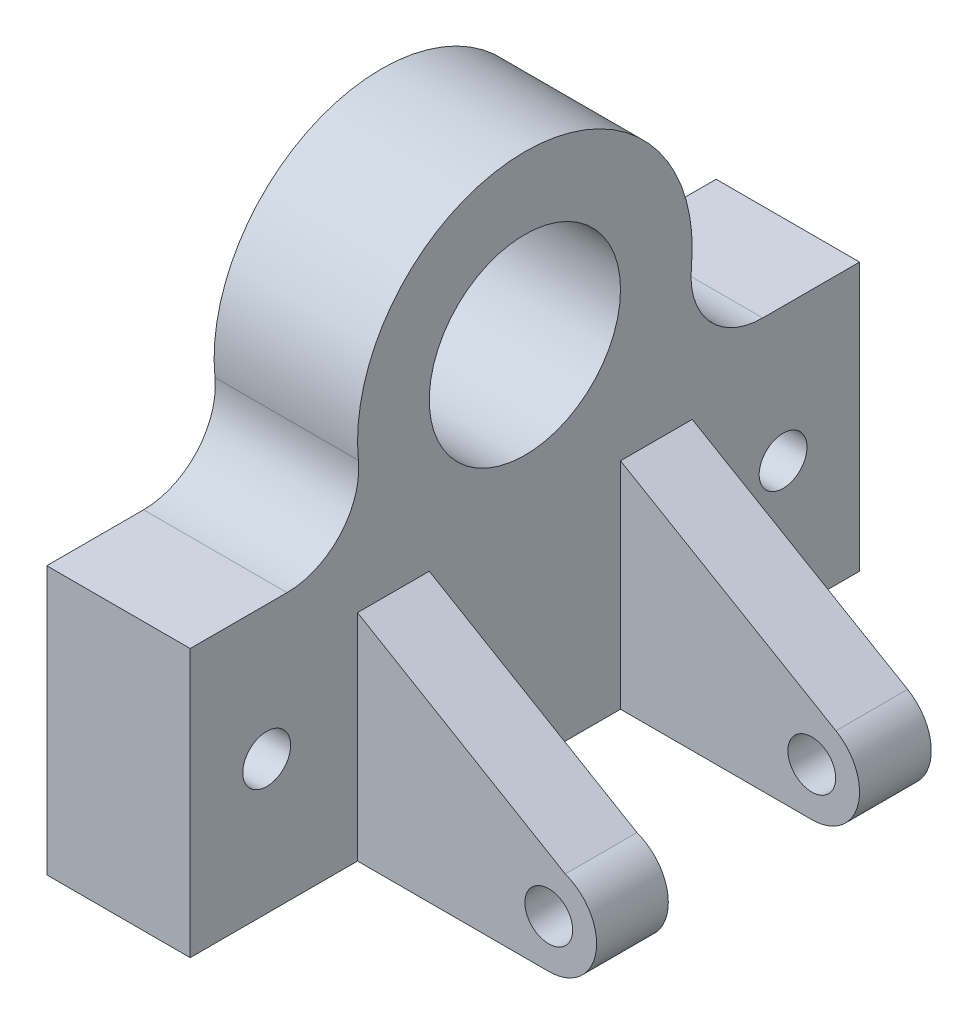
ISO-10303-21;
HEADER;
FILE_DESCRIPTION(('STEP AP214'),'2;1');
FILE_NAME('part.step','',(''),(''),'','','');
FILE_SCHEMA(('AUTOMOTIVE_DESIGN { 1 0 10303 214 1 1 1 1 }'));
ENDSEC;
DATA;
#1=APPLICATION_CONTEXT('core data for automotive mechanical design processes');
#2=APPLICATION_PROTOCOL_DEFINITION('international standard','automotive_design',2000,#1);
#3=PRODUCT_CONTEXT('',#1,'mechanical');
#4=PRODUCT('Part','Part','',(#3));
#5=PRODUCT_RELATED_PRODUCT_CATEGORY('part','',(#4));
#6=PRODUCT_DEFINITION_FORMATION('','',#4);
#7=PRODUCT_DEFINITION_CONTEXT('part definition',#1,'design');
#8=PRODUCT_DEFINITION('design','',#6,#7);
#9=PRODUCT_DEFINITION_SHAPE('','',#8);
#10=(LENGTH_UNIT() NAMED_UNIT(*) SI_UNIT(.MILLI.,.METRE.));
#11=(NAMED_UNIT(*) PLANE_ANGLE_UNIT() SI_UNIT($,.RADIAN.));
#12=(NAMED_UNIT(*) SI_UNIT($,.STERADIAN.) SOLID_ANGLE_UNIT());
#13=UNCERTAINTY_MEASURE_WITH_UNIT(LENGTH_MEASURE(1.E-05),#10,'distance_accuracy_value','');
#14=(GEOMETRIC_REPRESENTATION_CONTEXT(3) GLOBAL_UNCERTAINTY_ASSIGNED_CONTEXT((#13)) GLOBAL_UNIT_ASSIGNED_CONTEXT((#10,
#11,#12)) REPRESENTATION_CONTEXT('',''));
#15=CARTESIAN_POINT('',(0.,0.,0.));
#16=DIRECTION('',(0.,0.,1.));
#17=DIRECTION('',(1.,0.,0.));
#18=AXIS2_PLACEMENT_3D('',#15,#16,#17);
#19=CARTESIAN_POINT('',(15.,71.,-49.749371855331));
#20=DIRECTION('',(1.,0.,0.));
#21=DIRECTION('',(0.,0.,-1.));
#22=AXIS2_PLACEMENT_3D('',#19,#20,#21);
#23=PLANE('',#22);
#24=CARTESIAN_POINT('',(15.,76.,0.));
#25=DIRECTION('',(1.,0.,0.));
#26=DIRECTION('',(0.,0.,-1.));
#27=AXIS2_PLACEMENT_3D('',#24,#25,#26);
#28=CIRCLE('',#27,20.);
#29=CARTESIAN_POINT('',(15.,76.,-20.));
#30=VERTEX_POINT('',#29);
#31=EDGE_CURVE('E715',#30,#30,#28,.T.);
#32=ORIENTED_EDGE('',*,*,#31,.F.);
#33=EDGE_LOOP('',(#32));
#34=FACE_BOUND('',#33,.T.);
#35=CARTESIAN_POINT('',(15.,28.,54.));
#36=DIRECTION('',(1.,0.,0.));
#37=DIRECTION('',(0.,0.,-1.));
#38=AXIS2_PLACEMENT_3D('',#35,#36,#37);
#39=CIRCLE('',#38,5.);
#40=CARTESIAN_POINT('',(15.,28.,49.));
#41=VERTEX_POINT('',#40);
#42=EDGE_CURVE('E288',#41,#41,#39,.T.);
#43=ORIENTED_EDGE('',*,*,#42,.F.);
#44=EDGE_LOOP('',(#43));
#45=FACE_BOUND('',#44,.T.);
#46=CARTESIAN_POINT('',(15.,28.,-54.));
#47=DIRECTION('',(1.,0.,0.));
#48=DIRECTION('',(0.,0.,-1.));
#49=AXIS2_PLACEMENT_3D('',#46,#47,#48);
#50=CIRCLE('',#49,5.);
#51=CARTESIAN_POINT('',(15.,28.,-59.));
#52=VERTEX_POINT('',#51);
#53=EDGE_CURVE('E296',#52,#52,#50,.T.);
#54=ORIENTED_EDGE('',*,*,#53,.F.);
#55=EDGE_LOOP('',(#54));
#56=FACE_BOUND('',#55,.T.);
#57=DIRECTION('',(0.,0.,1.));
#58=VECTOR('',#57,1.);
#59=CARTESIAN_POINT('',(15.,45.,-35.));
#60=LINE('',#59,#58);
#61=CARTESIAN_POINT('',(15.,45.,-35.));
#62=VERTEX_POINT('',#61);
#63=CARTESIAN_POINT('',(15.,45.,-20.));
#64=VERTEX_POINT('',#63);
#65=EDGE_CURVE('E62',#62,#64,#60,.T.);
#66=ORIENTED_EDGE('',*,*,#65,.F.);
#67=DIRECTION('',(0.,-1.,0.));
#68=VECTOR('',#67,1.);
#69=CARTESIAN_POINT('',(15.,45.,-35.));
#70=LINE('',#69,#68);
#71=CARTESIAN_POINT('',(15.,0.,-35.));
#72=VERTEX_POINT('',#71);
#73=EDGE_CURVE('E169',#62,#72,#70,.T.);
#74=ORIENTED_EDGE('',*,*,#73,.T.);
#75=DIRECTION('',(0.,0.,-1.));
#76=VECTOR('',#75,1.);
#77=CARTESIAN_POINT('',(15.,0.,0.));
#78=LINE('',#77,#76);
#79=CARTESIAN_POINT('',(15.,0.,-70.));
#80=VERTEX_POINT('',#79);
#81=EDGE_CURVE('E157',#72,#80,#78,.T.);
#82=ORIENTED_EDGE('',*,*,#81,.T.);
#83=DIRECTION('',(0.,1.,0.));
#84=VECTOR('',#83,1.);
#85=CARTESIAN_POINT('',(15.,0.,-70.));
#86=LINE('',#85,#84);
#87=CARTESIAN_POINT('',(15.,56.,-70.));
#88=VERTEX_POINT('',#87);
#89=EDGE_CURVE('E228',#80,#88,#86,.T.);
#90=ORIENTED_EDGE('',*,*,#89,.T.);
#91=DIRECTION('',(0.,0.,1.));
#92=VECTOR('',#91,1.);
#93=CARTESIAN_POINT('',(15.,56.,-49.749371855331));
#94=LINE('',#93,#92);
#95=CARTESIAN_POINT('',(15.,56.,-49.749371855331));
#96=VERTEX_POINT('',#95);
#97=EDGE_CURVE('E233',#88,#96,#94,.T.);
#98=ORIENTED_EDGE('',*,*,#97,.T.);
#99=CARTESIAN_POINT('',(15.,71.,-49.749371855331));
#100=DIRECTION('',(-1.,0.,0.));
#101=DIRECTION('',(0.,0.,-1.));
#102=AXIS2_PLACEMENT_3D('',#99,#100,#101);
#103=CIRCLE('',#102,15.);
#104=CARTESIAN_POINT('',(15.,72.5,-34.8245602987317));
#105=VERTEX_POINT('',#104);
#106=EDGE_CURVE('E231',#96,#105,#103,.T.);
#107=ORIENTED_EDGE('',*,*,#106,.T.);
#108=CARTESIAN_POINT('',(15.,76.,0.));
#109=DIRECTION('',(1.,0.,0.));
#110=DIRECTION('',(0.,0.,-1.));
#111=AXIS2_PLACEMENT_3D('',#108,#109,#110);
#112=CIRCLE('',#111,35.);
#113=CARTESIAN_POINT('',(15.,72.5,34.8245602987317));
#114=VERTEX_POINT('',#113);
#115=EDGE_CURVE('E232',#105,#114,#112,.T.);
#116=ORIENTED_EDGE('',*,*,#115,.T.);
#117=CARTESIAN_POINT('',(15.,71.,49.749371855331));
#118=DIRECTION('',(-1.,0.,0.));
#119=DIRECTION('',(0.,0.,-1.));
#120=AXIS2_PLACEMENT_3D('',#117,#118,#119);
#121=CIRCLE('',#120,15.);
#122=CARTESIAN_POINT('',(15.,56.,49.749371855331));
#123=VERTEX_POINT('',#122);
#124=EDGE_CURVE('E240',#114,#123,#121,.T.);
#125=ORIENTED_EDGE('',*,*,#124,.T.);
#126=DIRECTION('',(0.,0.,1.));
#127=VECTOR('',#126,1.);
#128=CARTESIAN_POINT('',(15.,56.,70.));
#129=LINE('',#128,#127);
#130=CARTESIAN_POINT('',(15.,56.,70.));
#131=VERTEX_POINT('',#130);
#132=EDGE_CURVE('E239',#123,#131,#129,.T.);
#133=ORIENTED_EDGE('',*,*,#132,.T.);
#134=DIRECTION('',(0.,-1.,0.));
#135=VECTOR('',#134,1.);
#136=CARTESIAN_POINT('',(15.,0.,70.));
#137=LINE('',#136,#135);
#138=CARTESIAN_POINT('',(15.,0.,70.));
#139=VERTEX_POINT('',#138);
#140=EDGE_CURVE('E241',#131,#139,#137,.T.);
#141=ORIENTED_EDGE('',*,*,#140,.T.);
#142=CARTESIAN_POINT('',(15.,0.,35.));
#143=VERTEX_POINT('',#142);
#144=EDGE_CURVE('E170',#139,#143,#78,.T.);
#145=ORIENTED_EDGE('',*,*,#144,.T.);
#146=DIRECTION('',(0.,-1.,0.));
#147=VECTOR('',#146,1.);
#148=CARTESIAN_POINT('',(15.,0.,35.));
#149=LINE('',#148,#147);
#150=CARTESIAN_POINT('',(15.,45.,35.));
#151=VERTEX_POINT('',#150);
#152=EDGE_CURVE('E199',#151,#143,#149,.T.);
#153=ORIENTED_EDGE('',*,*,#152,.F.);
#154=DIRECTION('',(0.,0.,-1.));
#155=VECTOR('',#154,1.);
#156=CARTESIAN_POINT('',(15.,45.,35.));
#157=LINE('',#156,#155);
#158=CARTESIAN_POINT('',(15.,45.,20.));
#159=VERTEX_POINT('',#158);
#160=EDGE_CURVE('E209',#151,#159,#157,.T.);
#161=ORIENTED_EDGE('',*,*,#160,.T.);
#162=DIRECTION('',(0.,-1.,0.));
#163=VECTOR('',#162,1.);
#164=CARTESIAN_POINT('',(15.,0.,20.));
#165=LINE('',#164,#163);
#166=CARTESIAN_POINT('',(15.,0.,20.));
#167=VERTEX_POINT('',#166);
#168=EDGE_CURVE('E198',#159,#167,#165,.T.);
#169=ORIENTED_EDGE('',*,*,#168,.T.);
#170=CARTESIAN_POINT('',(15.,0.,-20.));
#171=VERTEX_POINT('',#170);
#172=EDGE_CURVE('E163',#167,#171,#78,.T.);
#173=ORIENTED_EDGE('',*,*,#172,.T.);
#174=DIRECTION('',(0.,-1.,0.));
#175=VECTOR('',#174,1.);
#176=CARTESIAN_POINT('',(15.,45.,-20.));
#177=LINE('',#176,#175);
#178=EDGE_CURVE('E70',#64,#171,#177,.T.);
#179=ORIENTED_EDGE('',*,*,#178,.F.);
#180=EDGE_LOOP('',(#66,#74,#82,#90,#98,#107,#116,#125,#133,#141,#145,#153,#161,#169,#173,#179));
#181=FACE_BOUND('',#180,.T.);
#182=ADVANCED_FACE('F44',(#34,#45,#56,#181),#23,.T.);
#183=CARTESIAN_POINT('',(15.,0.,-70.));
#184=DIRECTION('',(0.,0.,1.));
#185=DIRECTION('',(1.,0.,0.));
#186=AXIS2_PLACEMENT_3D('',#183,#184,#185);
#187=PLANE('',#186);
#188=DIRECTION('',(0.,1.,0.));
#189=VECTOR('',#188,1.);
#190=CARTESIAN_POINT('',(-15.,0.,-70.));
#191=LINE('',#190,#189);
#192=CARTESIAN_POINT('',(-15.,0.,-70.));
#193=VERTEX_POINT('',#192);
#194=CARTESIAN_POINT('',(-15.,56.,-70.));
#195=VERTEX_POINT('',#194);
#196=EDGE_CURVE('E226',#193,#195,#191,.T.);
#197=ORIENTED_EDGE('',*,*,#196,.T.);
#198=DIRECTION('',(-1.,0.,0.));
#199=VECTOR('',#198,1.);
#200=CARTESIAN_POINT('',(15.,56.,-70.));
#201=LINE('',#200,#199);
#202=EDGE_CURVE('E53',#88,#195,#201,.T.);
#203=ORIENTED_EDGE('',*,*,#202,.F.);
#204=ORIENTED_EDGE('',*,*,#89,.F.);
#205=DIRECTION('',(-1.,0.,0.));
#206=VECTOR('',#205,1.);
#207=CARTESIAN_POINT('',(15.,0.,-70.));
#208=LINE('',#207,#206);
#209=EDGE_CURVE('E11',#80,#193,#208,.T.);
#210=ORIENTED_EDGE('',*,*,#209,.T.);
#211=EDGE_LOOP('',(#197,#203,#204,#210));
#212=FACE_BOUND('',#211,.T.);
#213=ADVANCED_FACE('F50',(#212),#187,.F.);
#214=CARTESIAN_POINT('',(15.,56.,-49.749371855331));
#215=DIRECTION('',(0.,-1.,0.));
#216=DIRECTION('',(0.,0.,-1.));
#217=AXIS2_PLACEMENT_3D('',#214,#215,#216);
#218=PLANE('',#217);
#219=DIRECTION('',(0.,0.,1.));
#220=VECTOR('',#219,1.);
#221=CARTESIAN_POINT('',(-15.,56.,-49.749371855331));
#222=LINE('',#221,#220);
#223=CARTESIAN_POINT('',(-15.,56.,-49.749371855331));
#224=VERTEX_POINT('',#223);
#225=EDGE_CURVE('E248',#195,#224,#222,.T.);
#226=ORIENTED_EDGE('',*,*,#225,.T.);
#227=DIRECTION('',(-1.,0.,0.));
#228=VECTOR('',#227,1.);
#229=CARTESIAN_POINT('',(15.,56.,-49.749371855331));
#230=LINE('',#229,#228);
#231=EDGE_CURVE('E272',#96,#224,#230,.T.);
#232=ORIENTED_EDGE('',*,*,#231,.F.);
#233=ORIENTED_EDGE('',*,*,#97,.F.);
#234=ORIENTED_EDGE('',*,*,#202,.T.);
#235=EDGE_LOOP('',(#226,#232,#233,#234));
#236=FACE_BOUND('',#235,.T.);
#237=ADVANCED_FACE('F351',(#236),#218,.F.);
#238=CARTESIAN_POINT('',(15.,71.,-49.749371855331));
#239=DIRECTION('',(-1.,0.,0.));
#240=DIRECTION('',(0.,0.,1.));
#241=AXIS2_PLACEMENT_3D('',#238,#239,#240);
#242=CYLINDRICAL_SURFACE('',#241,15.);
#243=CARTESIAN_POINT('',(-15.,71.,-49.749371855331));
#244=DIRECTION('',(-1.,0.,0.));
#245=DIRECTION('',(0.,0.,-1.));
#246=AXIS2_PLACEMENT_3D('',#243,#244,#245);
#247=CIRCLE('',#246,15.);
#248=CARTESIAN_POINT('',(-15.,72.5,-34.8245602987317));
#249=VERTEX_POINT('',#248);
#250=EDGE_CURVE('E246',#224,#249,#247,.T.);
#251=ORIENTED_EDGE('',*,*,#250,.T.);
#252=DIRECTION('',(-1.,0.,0.));
#253=VECTOR('',#252,1.);
#254=CARTESIAN_POINT('',(15.,72.5,-34.8245602987317));
#255=LINE('',#254,#253);
#256=EDGE_CURVE('E269',#105,#249,#255,.T.);
#257=ORIENTED_EDGE('',*,*,#256,.F.);
#258=ORIENTED_EDGE('',*,*,#106,.F.);
#259=ORIENTED_EDGE('',*,*,#231,.T.);
#260=EDGE_LOOP('',(#251,#257,#258,#259));
#261=FACE_BOUND('',#260,.T.);
#262=ADVANCED_FACE('F377',(#261),#242,.F.);
#263=CARTESIAN_POINT('',(15.,76.,0.));
#264=DIRECTION('',(-1.,0.,0.));
#265=DIRECTION('',(0.,0.,1.));
#266=AXIS2_PLACEMENT_3D('',#263,#264,#265);
#267=CYLINDRICAL_SURFACE('',#266,35.);
#268=CARTESIAN_POINT('',(-15.,76.,0.));
#269=DIRECTION('',(1.,0.,0.));
#270=DIRECTION('',(0.,0.,-1.));
#271=AXIS2_PLACEMENT_3D('',#268,#269,#270);
#272=CIRCLE('',#271,35.);
#273=CARTESIAN_POINT('',(-15.,72.5,34.8245602987317));
#274=VERTEX_POINT('',#273);
#275=EDGE_CURVE('E247',#249,#274,#272,.T.);
#276=ORIENTED_EDGE('',*,*,#275,.T.);
#277=DIRECTION('',(-1.,0.,0.));
#278=VECTOR('',#277,1.);
#279=CARTESIAN_POINT('',(15.,72.5,34.8245602987317));
#280=LINE('',#279,#278);
#281=EDGE_CURVE('E270',#114,#274,#280,.T.);
#282=ORIENTED_EDGE('',*,*,#281,.F.);
#283=ORIENTED_EDGE('',*,*,#115,.F.);
#284=ORIENTED_EDGE('',*,*,#256,.T.);
#285=EDGE_LOOP('',(#276,#282,#283,#284));
#286=FACE_BOUND('',#285,.T.);
#287=ADVANCED_FACE('F374',(#286),#267,.T.);
#288=CARTESIAN_POINT('',(15.,71.,49.749371855331));
#289=DIRECTION('',(-1.,0.,0.));
#290=DIRECTION('',(0.,0.,1.));
#291=AXIS2_PLACEMENT_3D('',#288,#289,#290);
#292=CYLINDRICAL_SURFACE('',#291,15.);
#293=CARTESIAN_POINT('',(-15.,71.,49.749371855331));
#294=DIRECTION('',(-1.,0.,0.));
#295=DIRECTION('',(0.,0.,-1.));
#296=AXIS2_PLACEMENT_3D('',#293,#294,#295);
#297=CIRCLE('',#296,15.);
#298=CARTESIAN_POINT('',(-15.,56.,49.749371855331));
#299=VERTEX_POINT('',#298);
#300=EDGE_CURVE('E252',#274,#299,#297,.T.);
#301=ORIENTED_EDGE('',*,*,#300,.T.);
#302=DIRECTION('',(-1.,0.,0.));
#303=VECTOR('',#302,1.);
#304=CARTESIAN_POINT('',(15.,56.,49.749371855331));
#305=LINE('',#304,#303);
#306=EDGE_CURVE('E262',#123,#299,#305,.T.);
#307=ORIENTED_EDGE('',*,*,#306,.F.);
#308=ORIENTED_EDGE('',*,*,#124,.F.);
#309=ORIENTED_EDGE('',*,*,#281,.T.);
#310=EDGE_LOOP('',(#301,#307,#308,#309));
#311=FACE_BOUND('',#310,.T.);
#312=ADVANCED_FACE('F371',(#311),#292,.F.);
#313=CARTESIAN_POINT('',(15.,56.,70.));
#314=DIRECTION('',(0.,-1.,0.));
#315=DIRECTION('',(0.,0.,-1.));
#316=AXIS2_PLACEMENT_3D('',#313,#314,#315);
#317=PLANE('',#316);
#318=DIRECTION('',(0.,0.,1.));
#319=VECTOR('',#318,1.);
#320=CARTESIAN_POINT('',(-15.,56.,70.));
#321=LINE('',#320,#319);
#322=CARTESIAN_POINT('',(-15.,56.,70.));
#323=VERTEX_POINT('',#322);
#324=EDGE_CURVE('E255',#299,#323,#321,.T.);
#325=ORIENTED_EDGE('',*,*,#324,.T.);
#326=DIRECTION('',(-1.,0.,0.));
#327=VECTOR('',#326,1.);
#328=CARTESIAN_POINT('',(15.,56.,70.));
#329=LINE('',#328,#327);
#330=EDGE_CURVE('E261',#131,#323,#329,.T.);
#331=ORIENTED_EDGE('',*,*,#330,.F.);
#332=ORIENTED_EDGE('',*,*,#132,.F.);
#333=ORIENTED_EDGE('',*,*,#306,.T.);
#334=EDGE_LOOP('',(#325,#331,#332,#333));
#335=FACE_BOUND('',#334,.T.);
#336=ADVANCED_FACE('F370',(#335),#317,.F.);
#337=CARTESIAN_POINT('',(15.,0.,70.));
#338=DIRECTION('',(0.,0.,-1.));
#339=DIRECTION('',(-1.,0.,0.));
#340=AXIS2_PLACEMENT_3D('',#337,#338,#339);
#341=PLANE('',#340);
#342=DIRECTION('',(0.,-1.,0.));
#343=VECTOR('',#342,1.);
#344=CARTESIAN_POINT('',(-15.,0.,70.));
#345=LINE('',#344,#343);
#346=CARTESIAN_POINT('',(-15.,0.,70.));
#347=VERTEX_POINT('',#346);
#348=EDGE_CURVE('E258',#323,#347,#345,.T.);
#349=ORIENTED_EDGE('',*,*,#348,.T.);
#350=DIRECTION('',(-1.,0.,0.));
#351=VECTOR('',#350,1.);
#352=CARTESIAN_POINT('',(15.,0.,70.));
#353=LINE('',#352,#351);
#354=EDGE_CURVE('E243',#139,#347,#353,.T.);
#355=ORIENTED_EDGE('',*,*,#354,.F.);
#356=ORIENTED_EDGE('',*,*,#140,.F.);
#357=ORIENTED_EDGE('',*,*,#330,.T.);
#358=EDGE_LOOP('',(#349,#355,#356,#357));
#359=FACE_BOUND('',#358,.T.);
#360=ADVANCED_FACE('F365',(#359),#341,.F.);
#361=CARTESIAN_POINT('',(15.,0.,0.));
#362=DIRECTION('',(0.,1.,0.));
#363=DIRECTION('',(0.,0.,1.));
#364=AXIS2_PLACEMENT_3D('',#361,#362,#363);
#365=PLANE('',#364);
#366=DIRECTION('',(0.,0.,-1.));
#367=VECTOR('',#366,1.);
#368=CARTESIAN_POINT('',(-15.,0.,0.));
#369=LINE('',#368,#367);
#370=EDGE_CURVE('E164',#347,#193,#369,.T.);
#371=ORIENTED_EDGE('',*,*,#370,.T.);
#372=ORIENTED_EDGE('',*,*,#209,.F.);
#373=ORIENTED_EDGE('',*,*,#81,.F.);
#374=DIRECTION('',(1.,0.,0.));
#375=VECTOR('',#374,1.);
#376=CARTESIAN_POINT('',(15.,0.,-35.));
#377=LINE('',#376,#375);
#378=CARTESIAN_POINT('',(55.,0.,-35.));
#379=VERTEX_POINT('',#378);
#380=EDGE_CURVE('E165',#72,#379,#377,.T.);
#381=ORIENTED_EDGE('',*,*,#380,.T.);
#382=DIRECTION('',(0.,0.,1.));
#383=VECTOR('',#382,1.);
#384=CARTESIAN_POINT('',(55.,0.,-35.));
#385=LINE('',#384,#383);
#386=CARTESIAN_POINT('',(55.,0.,-20.));
#387=VERTEX_POINT('',#386);
#388=EDGE_CURVE('E184',#379,#387,#385,.T.);
#389=ORIENTED_EDGE('',*,*,#388,.T.);
#390=DIRECTION('',(1.,0.,0.));
#391=VECTOR('',#390,1.);
#392=CARTESIAN_POINT('',(15.,0.,-20.));
#393=LINE('',#392,#391);
#394=EDGE_CURVE('E186',#171,#387,#393,.T.);
#395=ORIENTED_EDGE('',*,*,#394,.F.);
#396=ORIENTED_EDGE('',*,*,#172,.F.);
#397=DIRECTION('',(1.,0.,0.));
#398=VECTOR('',#397,1.);
#399=CARTESIAN_POINT('',(15.,0.,20.));
#400=LINE('',#399,#398);
#401=CARTESIAN_POINT('',(55.,0.,20.));
#402=VERTEX_POINT('',#401);
#403=EDGE_CURVE('E213',#167,#402,#400,.T.);
#404=ORIENTED_EDGE('',*,*,#403,.T.);
#405=DIRECTION('',(0.,0.,-1.));
#406=VECTOR('',#405,1.);
#407=CARTESIAN_POINT('',(55.,0.,35.));
#408=LINE('',#407,#406);
#409=CARTESIAN_POINT('',(55.,0.,35.));
#410=VERTEX_POINT('',#409);
#411=EDGE_CURVE('E221',#410,#402,#408,.T.);
#412=ORIENTED_EDGE('',*,*,#411,.F.);
#413=DIRECTION('',(1.,0.,0.));
#414=VECTOR('',#413,1.);
#415=CARTESIAN_POINT('',(15.,0.,35.));
#416=LINE('',#415,#414);
#417=EDGE_CURVE('E201',#143,#410,#416,.T.);
#418=ORIENTED_EDGE('',*,*,#417,.F.);
#419=ORIENTED_EDGE('',*,*,#144,.F.);
#420=ORIENTED_EDGE('',*,*,#354,.T.);
#421=EDGE_LOOP('',(#371,#372,#373,#381,#389,#395,#396,#404,#412,#418,#419,#420));
#422=FACE_BOUND('',#421,.T.);
#423=ADVANCED_FACE('F159',(#422),#365,.F.);
#424=CARTESIAN_POINT('',(-15.,71.,-49.749371855331));
#425=DIRECTION('',(1.,0.,0.));
#426=DIRECTION('',(0.,0.,-1.));
#427=AXIS2_PLACEMENT_3D('',#424,#425,#426);
#428=PLANE('',#427);
#429=CARTESIAN_POINT('',(-15.,76.,0.));
#430=DIRECTION('',(1.,0.,0.));
#431=DIRECTION('',(0.,0.,-1.));
#432=AXIS2_PLACEMENT_3D('',#429,#430,#431);
#433=CIRCLE('',#432,20.);
#434=CARTESIAN_POINT('',(-15.,76.,-20.));
#435=VERTEX_POINT('',#434);
#436=EDGE_CURVE('E47',#435,#435,#433,.T.);
#437=ORIENTED_EDGE('',*,*,#436,.T.);
#438=EDGE_LOOP('',(#437));
#439=FACE_BOUND('',#438,.T.);
#440=CARTESIAN_POINT('',(-15.,28.,54.));
#441=DIRECTION('',(1.,0.,0.));
#442=DIRECTION('',(0.,0.,-1.));
#443=AXIS2_PLACEMENT_3D('',#440,#441,#442);
#444=CIRCLE('',#443,5.);
#445=CARTESIAN_POINT('',(-15.,28.,49.));
#446=VERTEX_POINT('',#445);
#447=EDGE_CURVE('E285',#446,#446,#444,.T.);
#448=ORIENTED_EDGE('',*,*,#447,.T.);
#449=EDGE_LOOP('',(#448));
#450=FACE_BOUND('',#449,.T.);
#451=CARTESIAN_POINT('',(-15.,28.,-54.));
#452=DIRECTION('',(1.,0.,0.));
#453=DIRECTION('',(0.,0.,-1.));
#454=AXIS2_PLACEMENT_3D('',#451,#452,#453);
#455=CIRCLE('',#454,5.);
#456=CARTESIAN_POINT('',(-15.,28.,-59.));
#457=VERTEX_POINT('',#456);
#458=EDGE_CURVE('E284',#457,#457,#455,.T.);
#459=ORIENTED_EDGE('',*,*,#458,.T.);
#460=EDGE_LOOP('',(#459));
#461=FACE_BOUND('',#460,.T.);
#462=ORIENTED_EDGE('',*,*,#196,.F.);
#463=ORIENTED_EDGE('',*,*,#370,.F.);
#464=ORIENTED_EDGE('',*,*,#348,.F.);
#465=ORIENTED_EDGE('',*,*,#324,.F.);
#466=ORIENTED_EDGE('',*,*,#300,.F.);
#467=ORIENTED_EDGE('',*,*,#275,.F.);
#468=ORIENTED_EDGE('',*,*,#250,.F.);
#469=ORIENTED_EDGE('',*,*,#225,.F.);
#470=EDGE_LOOP('',(#462,#463,#464,#465,#466,#467,#468,#469));
#471=FACE_BOUND('',#470,.T.);
#472=ADVANCED_FACE('F356',(#439,#450,#461,#471),#428,.F.);
#473=CARTESIAN_POINT('',(55.,10.,35.));
#474=DIRECTION('',(0.,0.,-1.));
#475=DIRECTION('',(-1.,0.,0.));
#476=AXIS2_PLACEMENT_3D('',#473,#474,#475);
#477=CYLINDRICAL_SURFACE('',#476,10.);
#478=CARTESIAN_POINT('',(55.,10.,20.));
#479=DIRECTION('',(0.,0.,1.));
#480=DIRECTION('',(1.,0.,0.));
#481=AXIS2_PLACEMENT_3D('',#478,#479,#480);
#482=CIRCLE('',#481,10.);
#483=CARTESIAN_POINT('',(58.4497590480061,19.3861154111112,20.));
#484=VERTEX_POINT('',#483);
#485=EDGE_CURVE('E214',#402,#484,#482,.T.);
#486=ORIENTED_EDGE('',*,*,#485,.T.);
#487=DIRECTION('',(0.,0.,-1.));
#488=VECTOR('',#487,1.);
#489=CARTESIAN_POINT('',(58.4497590480061,19.3861154111112,35.));
#490=LINE('',#489,#488);
#491=CARTESIAN_POINT('',(58.4497590480061,19.3861154111112,35.));
#492=VERTEX_POINT('',#491);
#493=EDGE_CURVE('E222',#492,#484,#490,.T.);
#494=ORIENTED_EDGE('',*,*,#493,.F.);
#495=CARTESIAN_POINT('',(55.,10.,35.));
#496=DIRECTION('',(0.,0.,1.));
#497=DIRECTION('',(1.,0.,0.));
#498=AXIS2_PLACEMENT_3D('',#495,#496,#497);
#499=CIRCLE('',#498,10.);
#500=EDGE_CURVE('E206',#410,#492,#499,.T.);
#501=ORIENTED_EDGE('',*,*,#500,.F.);
#502=ORIENTED_EDGE('',*,*,#411,.T.);
#503=EDGE_LOOP('',(#486,#494,#501,#502));
#504=FACE_BOUND('',#503,.T.);
#505=ADVANCED_FACE('F323',(#504),#477,.T.);
#506=CARTESIAN_POINT('',(15.,45.,35.));
#507=DIRECTION('',(-0.507833021256373,-0.861455525562187,0.));
#508=DIRECTION('',(0.861455525562188,-0.507833021256373,0.));
#509=AXIS2_PLACEMENT_3D('',#506,#507,#508);
#510=PLANE('',#509);
#511=DIRECTION('',(-0.861455525562187,0.507833021256373,0.));
#512=VECTOR('',#511,1.);
#513=CARTESIAN_POINT('',(15.,45.,20.));
#514=LINE('',#513,#512);
#515=EDGE_CURVE('E204',#484,#159,#514,.T.);
#516=ORIENTED_EDGE('',*,*,#515,.T.);
#517=ORIENTED_EDGE('',*,*,#160,.F.);
#518=DIRECTION('',(-0.861455525562187,0.507833021256373,0.));
#519=VECTOR('',#518,1.);
#520=CARTESIAN_POINT('',(15.,45.,35.));
#521=LINE('',#520,#519);
#522=EDGE_CURVE('E208',#492,#151,#521,.T.);
#523=ORIENTED_EDGE('',*,*,#522,.F.);
#524=ORIENTED_EDGE('',*,*,#493,.T.);
#525=EDGE_LOOP('',(#516,#517,#523,#524));
#526=FACE_BOUND('',#525,.T.);
#527=ADVANCED_FACE('F310',(#526),#510,.F.);
#528=CARTESIAN_POINT('',(55.,10.,35.));
#529=DIRECTION('',(0.,0.,1.));
#530=DIRECTION('',(1.,0.,0.));
#531=AXIS2_PLACEMENT_3D('',#528,#529,#530);
#532=PLANE('',#531);
#533=CARTESIAN_POINT('',(55.,10.,35.));
#534=DIRECTION('',(0.,0.,1.));
#535=DIRECTION('',(1.,0.,0.));
#536=AXIS2_PLACEMENT_3D('',#533,#534,#535);
#537=CIRCLE('',#536,5.);
#538=CARTESIAN_POINT('',(60.,10.,35.));
#539=VERTEX_POINT('',#538);
#540=EDGE_CURVE('E187',#539,#539,#537,.T.);
#541=ORIENTED_EDGE('',*,*,#540,.F.);
#542=EDGE_LOOP('',(#541));
#543=FACE_BOUND('',#542,.T.);
#544=ORIENTED_EDGE('',*,*,#152,.T.);
#545=ORIENTED_EDGE('',*,*,#417,.T.);
#546=ORIENTED_EDGE('',*,*,#500,.T.);
#547=ORIENTED_EDGE('',*,*,#522,.T.);
#548=EDGE_LOOP('',(#544,#545,#546,#547));
#549=FACE_BOUND('',#548,.T.);
#550=ADVANCED_FACE('F302',(#543,#549),#532,.T.);
#551=CARTESIAN_POINT('',(55.,10.,20.));
#552=DIRECTION('',(0.,0.,1.));
#553=DIRECTION('',(1.,0.,0.));
#554=AXIS2_PLACEMENT_3D('',#551,#552,#553);
#555=PLANE('',#554);
#556=CARTESIAN_POINT('',(55.,10.,20.));
#557=DIRECTION('',(0.,0.,1.));
#558=DIRECTION('',(1.,0.,0.));
#559=AXIS2_PLACEMENT_3D('',#556,#557,#558);
#560=CIRCLE('',#559,5.);
#561=CARTESIAN_POINT('',(60.,10.,20.));
#562=VERTEX_POINT('',#561);
#563=EDGE_CURVE('E281',#562,#562,#560,.T.);
#564=ORIENTED_EDGE('',*,*,#563,.T.);
#565=EDGE_LOOP('',(#564));
#566=FACE_BOUND('',#565,.T.);
#567=ORIENTED_EDGE('',*,*,#168,.F.);
#568=ORIENTED_EDGE('',*,*,#515,.F.);
#569=ORIENTED_EDGE('',*,*,#485,.F.);
#570=ORIENTED_EDGE('',*,*,#403,.F.);
#571=EDGE_LOOP('',(#567,#568,#569,#570));
#572=FACE_BOUND('',#571,.T.);
#573=ADVANCED_FACE('F306',(#566,#572),#555,.F.);
#574=CARTESIAN_POINT('',(60.0515173064048,18.630305493034,-35.));
#575=DIRECTION('',(0.505151730640476,0.863030549303402,0.));
#576=DIRECTION('',(-0.863030549303402,0.505151730640476,0.));
#577=AXIS2_PLACEMENT_3D('',#574,#575,#576);
#578=PLANE('',#577);
#579=DIRECTION('',(-0.863030549303402,0.505151730640476,0.));
#580=VECTOR('',#579,1.);
#581=CARTESIAN_POINT('',(60.0515173064048,18.630305493034,-20.));
#582=LINE('',#581,#580);
#583=CARTESIAN_POINT('',(60.0515173064048,18.630305493034,-20.));
#584=VERTEX_POINT('',#583);
#585=EDGE_CURVE('E172',#584,#64,#582,.T.);
#586=ORIENTED_EDGE('',*,*,#585,.F.);
#587=DIRECTION('',(0.,0.,1.));
#588=VECTOR('',#587,1.);
#589=CARTESIAN_POINT('',(60.0515173064048,18.630305493034,-35.));
#590=LINE('',#589,#588);
#591=CARTESIAN_POINT('',(60.0515173064048,18.630305493034,-35.));
#592=VERTEX_POINT('',#591);
#593=EDGE_CURVE('E197',#592,#584,#590,.T.);
#594=ORIENTED_EDGE('',*,*,#593,.F.);
#595=DIRECTION('',(-0.863030549303402,0.505151730640476,0.));
#596=VECTOR('',#595,1.);
#597=CARTESIAN_POINT('',(60.0515173064048,18.630305493034,-35.));
#598=LINE('',#597,#596);
#599=EDGE_CURVE('E179',#592,#62,#598,.T.);
#600=ORIENTED_EDGE('',*,*,#599,.T.);
#601=ORIENTED_EDGE('',*,*,#65,.T.);
#602=EDGE_LOOP('',(#586,#594,#600,#601));
#603=FACE_BOUND('',#602,.T.);
#604=ADVANCED_FACE('F334',(#603),#578,.T.);
#605=CARTESIAN_POINT('',(55.,10.,-35.));
#606=DIRECTION('',(0.,0.,1.));
#607=DIRECTION('',(1.,0.,0.));
#608=AXIS2_PLACEMENT_3D('',#605,#606,#607);
#609=CYLINDRICAL_SURFACE('',#608,10.);
#610=CARTESIAN_POINT('',(55.,10.,-20.));
#611=DIRECTION('',(0.,0.,1.));
#612=DIRECTION('',(1.,0.,0.));
#613=AXIS2_PLACEMENT_3D('',#610,#611,#612);
#614=CIRCLE('',#613,10.);
#615=EDGE_CURVE('E190',#387,#584,#614,.T.);
#616=ORIENTED_EDGE('',*,*,#615,.F.);
#617=ORIENTED_EDGE('',*,*,#388,.F.);
#618=CARTESIAN_POINT('',(55.,10.,-35.));
#619=DIRECTION('',(0.,0.,1.));
#620=DIRECTION('',(1.,0.,0.));
#621=AXIS2_PLACEMENT_3D('',#618,#619,#620);
#622=CIRCLE('',#621,10.);
#623=EDGE_CURVE('E180',#379,#592,#622,.T.);
#624=ORIENTED_EDGE('',*,*,#623,.T.);
#625=ORIENTED_EDGE('',*,*,#593,.T.);
#626=EDGE_LOOP('',(#616,#617,#624,#625));
#627=FACE_BOUND('',#626,.T.);
#628=ADVANCED_FACE('F333',(#627),#609,.T.);
#629=CARTESIAN_POINT('',(55.,10.,-35.));
#630=DIRECTION('',(0.,0.,1.));
#631=DIRECTION('',(1.,0.,0.));
#632=AXIS2_PLACEMENT_3D('',#629,#630,#631);
#633=PLANE('',#632);
#634=CARTESIAN_POINT('',(55.,10.,-35.));
#635=DIRECTION('',(0.,0.,-1.));
#636=DIRECTION('',(-1.,0.,0.));
#637=AXIS2_PLACEMENT_3D('',#634,#635,#636);
#638=CIRCLE('',#637,5.);
#639=CARTESIAN_POINT('',(50.,10.,-35.));
#640=VERTEX_POINT('',#639);
#641=EDGE_CURVE('E282',#640,#640,#638,.T.);
#642=ORIENTED_EDGE('',*,*,#641,.F.);
#643=EDGE_LOOP('',(#642));
#644=FACE_BOUND('',#643,.T.);
#645=ORIENTED_EDGE('',*,*,#73,.F.);
#646=ORIENTED_EDGE('',*,*,#599,.F.);
#647=ORIENTED_EDGE('',*,*,#623,.F.);
#648=ORIENTED_EDGE('',*,*,#380,.F.);
#649=EDGE_LOOP('',(#645,#646,#647,#648));
#650=FACE_BOUND('',#649,.T.);
#651=ADVANCED_FACE('F175',(#644,#650),#633,.F.);
#652=CARTESIAN_POINT('',(55.,10.,-20.));
#653=DIRECTION('',(0.,0.,1.));
#654=DIRECTION('',(1.,0.,0.));
#655=AXIS2_PLACEMENT_3D('',#652,#653,#654);
#656=PLANE('',#655);
#657=CARTESIAN_POINT('',(55.,10.,-20.));
#658=DIRECTION('',(0.,0.,1.));
#659=DIRECTION('',(1.,0.,0.));
#660=AXIS2_PLACEMENT_3D('',#657,#658,#659);
#661=CIRCLE('',#660,5.);
#662=CARTESIAN_POINT('',(60.,10.,-20.));
#663=VERTEX_POINT('',#662);
#664=EDGE_CURVE('E279',#663,#663,#661,.T.);
#665=ORIENTED_EDGE('',*,*,#664,.F.);
#666=EDGE_LOOP('',(#665));
#667=FACE_BOUND('',#666,.T.);
#668=ORIENTED_EDGE('',*,*,#178,.T.);
#669=ORIENTED_EDGE('',*,*,#394,.T.);
#670=ORIENTED_EDGE('',*,*,#615,.T.);
#671=ORIENTED_EDGE('',*,*,#585,.T.);
#672=EDGE_LOOP('',(#668,#669,#670,#671));
#673=FACE_BOUND('',#672,.T.);
#674=ADVANCED_FACE('F329',(#667,#673),#656,.T.);
#675=CARTESIAN_POINT('',(55.,10.,65.));
#676=DIRECTION('',(0.,0.,-1.));
#677=DIRECTION('',(-1.,0.,0.));
#678=AXIS2_PLACEMENT_3D('',#675,#676,#677);
#679=CYLINDRICAL_SURFACE('',#678,5.);
#680=ORIENTED_EDGE('',*,*,#664,.T.);
#681=EDGE_LOOP('',(#680));
#682=FACE_BOUND('',#681,.T.);
#683=ORIENTED_EDGE('',*,*,#641,.T.);
#684=EDGE_LOOP('',(#683));
#685=FACE_BOUND('',#684,.T.);
#686=ADVANCED_FACE('F477',(#682,#685),#679,.F.);
#687=ORIENTED_EDGE('',*,*,#540,.T.);
#688=EDGE_LOOP('',(#687));
#689=FACE_BOUND('',#688,.T.);
#690=ORIENTED_EDGE('',*,*,#563,.F.);
#691=EDGE_LOOP('',(#690));
#692=FACE_BOUND('',#691,.T.);
#693=ADVANCED_FACE('F305',(#689,#692),#679,.F.);
#694=CARTESIAN_POINT('',(-85.,28.,-54.));
#695=DIRECTION('',(1.,0.,0.));
#696=DIRECTION('',(0.,0.,-1.));
#697=AXIS2_PLACEMENT_3D('',#694,#695,#696);
#698=CYLINDRICAL_SURFACE('',#697,5.);
#699=ORIENTED_EDGE('',*,*,#53,.T.);
#700=EDGE_LOOP('',(#699));
#701=FACE_BOUND('',#700,.T.);
#702=ORIENTED_EDGE('',*,*,#458,.F.);
#703=EDGE_LOOP('',(#702));
#704=FACE_BOUND('',#703,.T.);
#705=ADVANCED_FACE('F501',(#701,#704),#698,.F.);
#706=CARTESIAN_POINT('',(-85.,28.,54.));
#707=DIRECTION('',(1.,0.,0.));
#708=DIRECTION('',(0.,0.,-1.));
#709=AXIS2_PLACEMENT_3D('',#706,#707,#708);
#710=CYLINDRICAL_SURFACE('',#709,5.);
#711=ORIENTED_EDGE('',*,*,#42,.T.);
#712=EDGE_LOOP('',(#711));
#713=FACE_BOUND('',#712,.T.);
#714=ORIENTED_EDGE('',*,*,#447,.F.);
#715=EDGE_LOOP('',(#714));
#716=FACE_BOUND('',#715,.T.);
#717=ADVANCED_FACE('F509',(#713,#716),#710,.F.);
#718=CARTESIAN_POINT('',(-85.,76.,0.));
#719=DIRECTION('',(1.,0.,0.));
#720=DIRECTION('',(0.,0.,-1.));
#721=AXIS2_PLACEMENT_3D('',#718,#719,#720);
#722=CYLINDRICAL_SURFACE('',#721,20.);
#723=ORIENTED_EDGE('',*,*,#31,.T.);
#724=EDGE_LOOP('',(#723));
#725=FACE_BOUND('',#724,.T.);
#726=ORIENTED_EDGE('',*,*,#436,.F.);
#727=EDGE_LOOP('',(#726));
#728=FACE_BOUND('',#727,.T.);
#729=ADVANCED_FACE('F519',(#725,#728),#722,.F.);
#730=CLOSED_SHELL('',(#182,#213,#237,#262,#287,#312,#336,#360,#423,#472,#505,#527,#550,#573,
#604,#628,#651,#674,#686,#693,#705,#717,#729));
#731=MANIFOLD_SOLID_BREP('B2',#730);
#732=ADVANCED_BREP_SHAPE_REPRESENTATION('',(#18,#731),#14);
#733=SHAPE_DEFINITION_REPRESENTATION(#9,#732);
ENDSEC;
END-ISO-10303-21;
